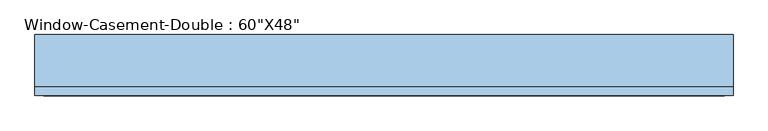
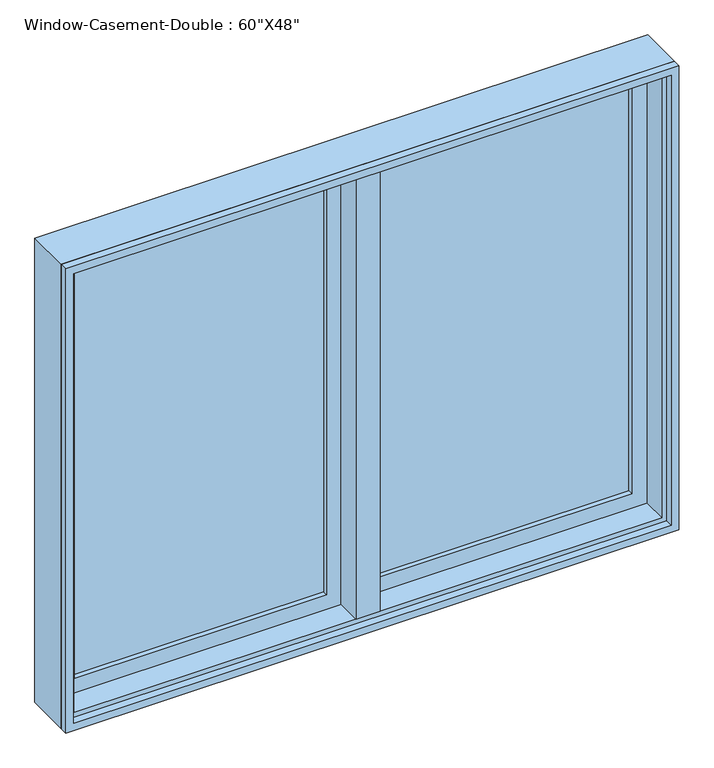
"""IFC4 building model written with IfcOpenShell, lengths in millimetres: window geometry."""

from ifc_helpers import new_model, si_unit, frame, origin, place, context, project, spatial, polyline, outline, extrude, faceted_brep, source, transform, mapped, element, save


def window_9418cf83(model_context):
    return source(origin(), model_context, "Body", "SolidModel", [
        faceted_brep([(9.525, 76.2, 2120.9), (-9.525, 76.2, 2120.9), (-9.525, 25.4, 2120.9), (9.525, 25.4, 2120.9), (9.525, 76.2, 927.1), (9.525, 25.4, 927.1), (-9.525, 25.4, 927.1), (-9.525, 76.2, 927.1), (-9.525, 25.4, 946.15), (-9.525, 25.4, 2101.85), (-30.1625, 25.4, 946.15), (-30.1625, 25.4, 2101.85), (-30.1625, -38.1, 946.15), (-30.1625, -38.1, 2101.85), (30.1625, -38.1, 946.15), (30.1625, -38.1, 2101.85), (30.1625, 25.4, 946.15), (30.1625, 25.4, 2101.85), (9.525, 25.4, 946.15), (9.525, 25.4, 2101.85)], [[[0, 1, 2, 3]], [[4, 5, 6, 7]], [[1, 0, 4, 7]], [[2, 1, 7, 6, 8, 9]], [[9, 8, 10, 11]], [[11, 10, 12, 13]], [[13, 12, 14, 15]], [[15, 14, 16, 17]], [[17, 16, 18, 19]], [[0, 3, 19, 18, 5, 4]], [[18, 8, 6, 5]], [[9, 19, 3, 2]], [[8, 18, 16, 14, 12, 10]], [[19, 9, 11, 13, 15, 17]]]),
        extrude(outline(polyline([(-66.675, 57.15), (-66.675, 50.8), (-692.15, 50.8), (-692.15, 57.15), (-66.675, 57.15)])), frame((0.0, 0.0, 984.25), z_axis=(0.0, 0.0, 1.0), x_axis=(1.0, 0.0, 0.0)), (0.0, 0.0, 1.0), 1079.5),
        extrude(outline(polyline([(-692.15, 38.1), (-692.15, 44.45), (-66.675, 44.45), (-66.675, 38.1), (-692.15, 38.1)])), frame((0.0, 0.0, 984.25), z_axis=(0.0, 0.0, 1.0), x_axis=(1.0, 0.0, 0.0)), (0.0, 0.0, 1.0), 1079.5),
        extrude(outline(polyline([(692.15, 57.15), (692.15, 50.8), (66.675, 50.8), (66.675, 57.15), (692.15, 57.15)])), frame((0.0, 0.0, 984.25), z_axis=(0.0, 0.0, 1.0), x_axis=(1.0, 0.0, 0.0)), (0.0, 0.0, 1.0), 1079.5),
        extrude(outline(polyline([(66.675, 38.1), (66.675, 44.45), (692.15, 44.45), (692.15, 38.1), (66.675, 38.1)])), frame((0.0, 0.0, 984.25), z_axis=(0.0, 0.0, 1.0), x_axis=(1.0, 0.0, 0.0)), (0.0, 0.0, 1.0), 1079.5),
        extrude(outline(polyline([(2120.9, -749.3), (927.1, -749.3), (927.1, -9.525), (2120.9, -9.525), (2120.9, -749.3)]), holes=[polyline([(2063.75, -66.675), (984.25, -66.675), (984.25, -692.15), (2063.75, -692.15), (2063.75, -66.675)])]), frame((0.0, 25.4, 0.0), z_axis=(0.0, 1.0, 0.0), x_axis=(0.0, 0.0, 1.0)), (0.0, 0.0, 1.0), 44.45),
        extrude(outline(polyline([(927.1, 749.3), (2120.9, 749.3), (2120.9, 9.525), (927.1, 9.525), (927.1, 749.3)]), holes=[polyline([(984.25, 66.675), (2063.75, 66.675), (2063.75, 692.15), (984.25, 692.15), (984.25, 66.675)])]), frame((0.0, 25.4, 0.0), z_axis=(0.0, 1.0, 0.0), x_axis=(0.0, 0.0, 1.0)), (0.0, 0.0, 1.0), 44.45),
        extrude(outline(polyline([(2133.6, -762.0), (914.4, -762.0), (914.4, 762.0), (2133.6, 762.0), (2133.6, -762.0)]), holes=[polyline([(2114.55, 742.95), (933.45, 742.95), (933.45, -742.95), (2114.55, -742.95), (2114.55, 742.95)])]), frame((0.0, -57.15, 0.0), z_axis=(0.0, 1.0, 0.0), x_axis=(0.0, 0.0, 1.0)), (0.0, 0.0, 1.0), 19.05),
        faceted_brep([(730.25, 25.4, 2101.85), (730.25, -38.1, 2101.85), (-730.25, -38.1, 2101.85), (-730.25, 25.4, 2101.85), (749.3, 76.2, 2120.9), (749.3, 25.4, 2120.9), (-749.3, 25.4, 2120.9), (-749.3, 76.2, 2120.9), (762.0, -38.1, 2133.6), (762.0, 76.2, 2133.6), (-762.0, 76.2, 2133.6), (-762.0, -38.1, 2133.6), (-730.25, -38.1, 946.15), (-730.25, 25.4, 946.15), (-749.3, 25.4, 927.1), (-749.3, 76.2, 927.1), (-762.0, 76.2, 914.4), (-762.0, -38.1, 914.4), (730.25, -38.1, 946.15), (730.25, 25.4, 946.15), (749.3, 25.4, 927.1), (749.3, 76.2, 927.1), (762.0, 76.2, 914.4), (762.0, -38.1, 914.4)], [[[0, 1, 2, 3]], [[4, 5, 6, 7]], [[8, 9, 10, 11]], [[3, 2, 12, 13]], [[7, 6, 14, 15]], [[11, 10, 16, 17]], [[13, 12, 18, 19]], [[15, 14, 20, 21]], [[17, 16, 22, 23]], [[11, 17, 23, 8], [1, 18, 12, 2]], [[19, 18, 1, 0]], [[5, 20, 14, 6], [3, 13, 19, 0]], [[21, 20, 5, 4]], [[23, 22, 9, 8]], [[9, 22, 16, 10], [7, 15, 21, 4]]]),
    ])


if __name__ == "__main__":
    model = new_model("IFC4")
    model_context = context("Model", 3, world=origin())
    ifc_project = project(units=[si_unit("LENGTHUNIT", "METRE", prefix="MILLI")], contexts=[model_context])
    site = spatial("IfcSite", under=ifc_project)
    building = spatial("IfcBuilding", under=site)
    placement = place(None, origin())
    window_shape = window_9418cf83(model_context)
    element("IfcWindow", 1, ObjectType="Window-Casement-Double : 60\"X48\"", at=placement, inside=building, context=model_context, shape_type="MappedRepresentation", body=[
        mapped(window_shape, transform((0.0, 0.0, 0.0), x_axis=(1.0, 0.0, 0.0), y_axis=(0.0, 1.0, 0.0), z_axis=(0.0, 0.0, 1.0))),
    ])
    save(model, "model.ifc")

# Revit data of these elements
# Type "Window-Casement-Double : 60\"X48\""
#   Type Mark = "W"
#   Fire Rating = "0.5h"
#   Assembly Code = "B2020100"
#   Analytic Construction = "Double glazing - domestic"
#   Frame Extension [instance default] = 0' - 0 1/4"
#   Window Inset [instance default] = 0' - 0"
#   Wall Thickness [instance default] = 0' - 6"
#   Interior Wall Closure [instance default] = 0' - 2 1/4"
#   Half Width = 2' - 6"
#   Visual Light Transmittance = 0.81
#   Thermal Resistance (R) = 1.8146 (h·ft²·°F)/BTU
#   Solar Heat Gain Coefficient = 0.76
#   Rough Width = 5' - 0 1/2"
#   Rough Height = 4' - 0 1/2"
#   Height = 4' - 0"
#   Heat Transfer Coefficient (U) = 0.5511 BTU/(h·ft²·°F)
#   Exterior Wall Closure [instance default] = 0' - 1 1/4"
#   Extension Jamb [instance default] = 0' - 2 1/4"
#   Default Sill Height = 3' - 0"
#   Width = 5' - 0"
#   Muntin Visibility = yes
#   Interior Trim Visibility [instance default] = yes
#   Exterior Trim Visibility [instance default] = yes
#   Extension Jamb Visibility [instance default] = yes
#   Interior Trim Material = Wood - Stained
#   Muntin Pattern = Muntin Pattern_2x2 : Muntin Pattern_2x2
#   Interior Trim = Trim-Window-Interior-Flat : Picture Frame
#   Interior Frame Material = Wood - Stained
#   Glass Panel Material = Glass
#   Exterior Trim Material = Clad - White
#   Exterior Trim = Trim-Window-Exterior-Flat : with Sill
#   Exterior Frame Material = Clad - White
#   Wall Closure = (empty or 0)
# Element 1 (IfcWindow, "Window-Casement-Double : 60\"X48\"")
#   Wall Thickness = 0' - 4 1/2"
#   Extension Jamb = 0' - 0 3/4"
#   Materials on its faces: "Wood - Stained", "Glass", "Clad - White"
# Materials
#   "Wood - Stained": class "Wood", colour RGB 224 178 126, transparency 0, Cost = 0
#   "Glass": class "Glass", colour RGB 0 128 192, transparency 0.75, Description = "Soda Lime Glass", Cost = 0
#   "Clad - White": class "Wood", colour RGB 242 242 238, transparency 0, Cost = 0
